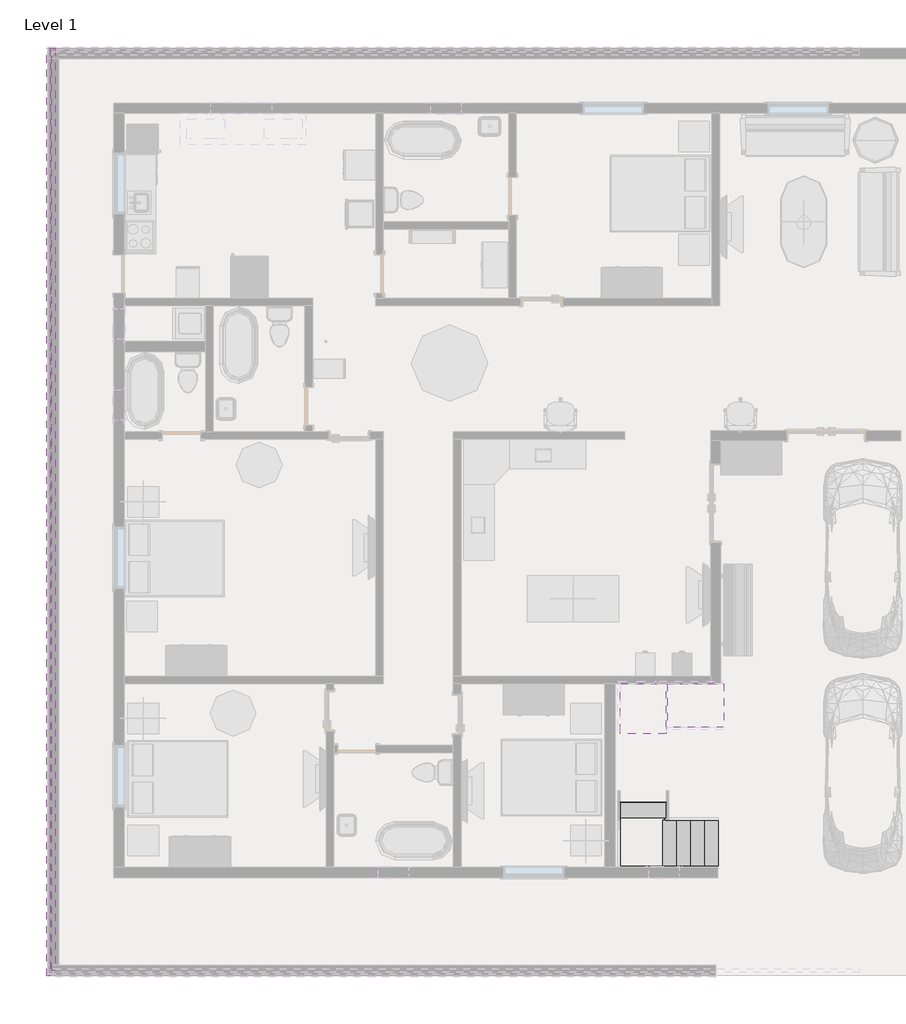
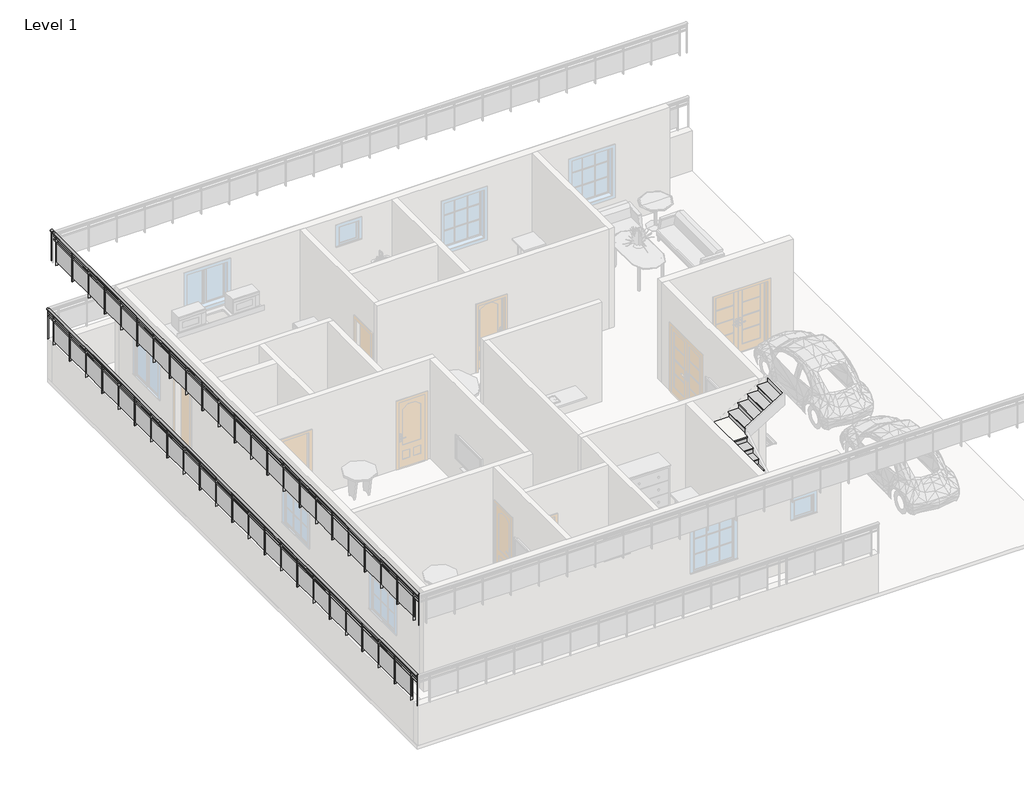
# One storey, part 3 of 6: 3 stair flights, 2 railings, 2 slabs.
"""IFC4 building model written with IfcOpenShell, lengths in millimetres."""

from ifc_helpers import new_model, si_unit, point, frame, origin, place, context, project, spatial, polyline, ellipse_curve, trimmed, outline, extrude, transform, mapped, element, save
from ifc_brep_helpers import plane_surface, extruded_surface, advanced_brep
from components import non_monolithic_landing_8bb0a33a, non_monolithic_landing_17065b0a, stair_flight_2df9e6b5, stair_flight_2e9a7ce1, stair_flight_c310d209

model = new_model("IFC4")

# Units and contexts
model_context = context("Model", 3, world=origin())
ifc_project = project(units=[si_unit("LENGTHUNIT", "METRE", prefix="MILLI")], contexts=[model_context])

# Site, building, storey
site = spatial("IfcSite", under=ifc_project)
building = spatial("IfcBuilding", under=site)
storey = spatial("IfcBuildingStorey", under=building, Name="Level 1", Elevation=0.0)

# Railings
placement = place(None, origin())
element("IfcRailing", 1, ObjectType="Glass Panel - Bottom Fill", at=placement, inside=storey, context=model_context, shape_type="SolidModel", body=[
    advanced_brep(
    [(-7851.6402326, 14000.8633056, 2133.6), (-7927.8402326, 14000.8633056, 2133.6), (-7851.6402326, -4490.3366944, 2133.6), (-7927.8402326, -4490.3366944, 2133.6)],
    [
        (0, 1, ellipse_curve(frame((-7889.7402326, 14000.8633056, 2133.6), z_axis=(0.0, 1.0, 0.0), x_axis=(-1.0, 0.0, 0.0)), 38.1, 28.575)),
        (1, 0, ellipse_curve(frame((-7889.7402326, 14000.8633056, 2133.6), z_axis=(0.0, 1.0, 0.0), x_axis=(-1.0, 0.0, 0.0)), 38.1, 28.575)),
        (2, 3, ellipse_curve(frame((-7889.7402326, -4490.3366944, 2133.6), z_axis=(0.0, -1.0, 0.0), x_axis=(-1.0, 0.0, 0.0)), 38.1, 28.575)),
        (3, 2, ellipse_curve(frame((-7889.7402326, -4490.3366944, 2133.6), z_axis=(0.0, -1.0, 0.0), x_axis=(-1.0, 0.0, 0.0)), 38.1, 28.575)),
        (0, 2),
        (3, 1),
    ],
    [
        plane_surface(frame((-7889.7402326, 14000.8633056, 2133.6), z_axis=(0.0, 1.0, 0.0), x_axis=(0.0, 0.0, -1.0))),
        plane_surface(frame((-7889.7402326, -4490.3366944, 2133.6), z_axis=(0.0, -1.0, 0.0), x_axis=(0.0, 0.0, -1.0))),
        extruded_surface(trimmed(ellipse_curve(frame((-7889.7402326, -4490.3366944, 2133.6), z_axis=(0.0, 1.0, 0.0), x_axis=(-1.0, 0.0, 0.0)), 38.1, 28.575), [point((-7851.6402326, -4490.3366944, 2133.6))], [point((-7927.8402326, -4490.3366944, 2133.6))], True, "CARTESIAN"), (0.0, 18491.2, 0.0), 18491.2),
        extruded_surface(trimmed(ellipse_curve(frame((-7889.7402326, -4490.3366944, 2133.6), z_axis=(0.0, 1.0, 0.0), x_axis=(-1.0, 0.0, 0.0)), 38.1, 28.575), [point((-7927.8402326, -4490.3366944, 2133.6))], [point((-7851.6402326, -4490.3366944, 2133.6))], True, "CARTESIAN"), (0.0, 18491.2, 0.0), 18491.2),
    ],
    [
        (0, [[1, 2]]),
        (1, [[3, 4]]),
        (2, [[-1, 5, -4, 6]]),
        (3, [[-2, -6, -3, -5]]),
    ],
),
    extrude(outline(polyline([(-7902.4402326, 14000.8633056), (-7877.0402326, 14000.8633056), (-7877.0402326, -4490.3366944), (-7902.4402326, -4490.3366944), (-7902.4402326, 14000.8633056)])), frame((0.0, 0.0, 2019.3), z_axis=(0.0, 0.0, 1.0), x_axis=(1.0, 0.0, 0.0)), (0.0, 0.0, 1.0), 25.4),
    extrude(outline(polyline([(-7902.4402326, 14000.8633056), (-7877.0402326, 14000.8633056), (-7877.0402326, -4490.3366944), (-7902.4402326, -4490.3366944), (-7902.4402326, 14000.8633056)])), frame((0.0, 0.0, 1917.7), z_axis=(0.0, 0.0, 1.0), x_axis=(1.0, 0.0, 0.0)), (0.0, 0.0, 1.0), 25.4),
    extrude(outline(polyline([(-7915.1402326, -4179.1866944), (-7864.3402326, -4179.1866944), (-7864.3402326, -4191.8866944), (-7915.1402326, -4191.8866944), (-7915.1402326, -4179.1866944)])), frame((0.0, 0.0, 1219.2), z_axis=(0.0, 0.0, 1.0), x_axis=(1.0, 0.0, 0.0)), (0.0, 0.0, 1.0), 885.6788223),
    extrude(outline(polyline([(-7883.2050756, -3372.7366944), (-7883.2050756, -4185.5366944), (-7889.5550756, -4185.5366944), (-7889.5550756, -3372.7366944), (-7883.2050756, -3372.7366944)])), frame((0.0, 0.0, 1320.8), z_axis=(0.0, 0.0, 1.0), x_axis=(1.0, 0.0, 0.0)), (0.0, 0.0, 1.0), 596.9),
    extrude(outline(polyline([(-7915.1402326, -3366.3866944), (-7864.3402326, -3366.3866944), (-7864.3402326, -3379.0866944), (-7915.1402326, -3379.0866944), (-7915.1402326, -3366.3866944)])), frame((0.0, 0.0, 1219.2), z_axis=(0.0, 0.0, 1.0), x_axis=(1.0, 0.0, 0.0)), (0.0, 0.0, 1.0), 885.6788223),
    extrude(outline(polyline([(-7883.2050756, -2559.9366944), (-7883.2050756, -3372.7366944), (-7889.5550756, -3372.7366944), (-7889.5550756, -2559.9366944), (-7883.2050756, -2559.9366944)])), frame((0.0, 0.0, 1320.8), z_axis=(0.0, 0.0, 1.0), x_axis=(1.0, 0.0, 0.0)), (0.0, 0.0, 1.0), 596.9),
    extrude(outline(polyline([(-7915.1402326, -2553.5866944), (-7864.3402326, -2553.5866944), (-7864.3402326, -2566.2866944), (-7915.1402326, -2566.2866944), (-7915.1402326, -2553.5866944)])), frame((0.0, 0.0, 1219.2), z_axis=(0.0, 0.0, 1.0), x_axis=(1.0, 0.0, 0.0)), (0.0, 0.0, 1.0), 885.6788223),
    extrude(outline(polyline([(-7883.2050756, -1747.1366944), (-7883.2050756, -2559.9366944), (-7889.5550756, -2559.9366944), (-7889.5550756, -1747.1366944), (-7883.2050756, -1747.1366944)])), frame((0.0, 0.0, 1320.8), z_axis=(0.0, 0.0, 1.0), x_axis=(1.0, 0.0, 0.0)), (0.0, 0.0, 1.0), 596.9),
    extrude(outline(polyline([(-7915.1402326, -1740.7866944), (-7864.3402326, -1740.7866944), (-7864.3402326, -1753.4866944), (-7915.1402326, -1753.4866944), (-7915.1402326, -1740.7866944)])), frame((0.0, 0.0, 1219.2), z_axis=(0.0, 0.0, 1.0), x_axis=(1.0, 0.0, 0.0)), (0.0, 0.0, 1.0), 885.6788223),
    extrude(outline(polyline([(-7883.2050756, -934.3366944), (-7883.2050756, -1747.1366944), (-7889.5550756, -1747.1366944), (-7889.5550756, -934.3366944), (-7883.2050756, -934.3366944)])), frame((0.0, 0.0, 1320.8), z_axis=(0.0, 0.0, 1.0), x_axis=(1.0, 0.0, 0.0)), (0.0, 0.0, 1.0), 596.9),
    extrude(outline(polyline([(-7915.1402326, -927.9866944), (-7864.3402326, -927.9866944), (-7864.3402326, -940.6866944), (-7915.1402326, -940.6866944), (-7915.1402326, -927.9866944)])), frame((0.0, 0.0, 1219.2), z_axis=(0.0, 0.0, 1.0), x_axis=(1.0, 0.0, 0.0)), (0.0, 0.0, 1.0), 885.6788223),
    extrude(outline(polyline([(-7883.2050756, -121.5366944), (-7883.2050756, -934.3366944), (-7889.5550756, -934.3366944), (-7889.5550756, -121.5366944), (-7883.2050756, -121.5366944)])), frame((0.0, 0.0, 1320.8), z_axis=(0.0, 0.0, 1.0), x_axis=(1.0, 0.0, 0.0)), (0.0, 0.0, 1.0), 596.9),
    extrude(outline(polyline([(-7915.1402326, -115.1866944), (-7864.3402326, -115.1866944), (-7864.3402326, -127.8866944), (-7915.1402326, -127.8866944), (-7915.1402326, -115.1866944)])), frame((0.0, 0.0, 1219.2), z_axis=(0.0, 0.0, 1.0), x_axis=(1.0, 0.0, 0.0)), (0.0, 0.0, 1.0), 885.6788223),
    extrude(outline(polyline([(-7883.2050756, 691.2633056), (-7883.2050756, -121.5366944), (-7889.5550756, -121.5366944), (-7889.5550756, 691.2633056), (-7883.2050756, 691.2633056)])), frame((0.0, 0.0, 1320.8), z_axis=(0.0, 0.0, 1.0), x_axis=(1.0, 0.0, 0.0)), (0.0, 0.0, 1.0), 596.9),
    extrude(outline(polyline([(-7915.1402326, 697.6133056), (-7864.3402326, 697.6133056), (-7864.3402326, 684.9133056), (-7915.1402326, 684.9133056), (-7915.1402326, 697.6133056)])), frame((0.0, 0.0, 1219.2), z_axis=(0.0, 0.0, 1.0), x_axis=(1.0, 0.0, 0.0)), (0.0, 0.0, 1.0), 885.6788223),
    extrude(outline(polyline([(-7883.2050756, 1504.0633056), (-7883.2050756, 691.2633056), (-7889.5550756, 691.2633056), (-7889.5550756, 1504.0633056), (-7883.2050756, 1504.0633056)])), frame((0.0, 0.0, 1320.8), z_axis=(0.0, 0.0, 1.0), x_axis=(1.0, 0.0, 0.0)), (0.0, 0.0, 1.0), 596.9),
    extrude(outline(polyline([(-7915.1402326, 1510.4133056), (-7864.3402326, 1510.4133056), (-7864.3402326, 1497.7133056), (-7915.1402326, 1497.7133056), (-7915.1402326, 1510.4133056)])), frame((0.0, 0.0, 1219.2), z_axis=(0.0, 0.0, 1.0), x_axis=(1.0, 0.0, 0.0)), (0.0, 0.0, 1.0), 885.6788223),
    extrude(outline(polyline([(-7883.2050756, 2316.8633056), (-7883.2050756, 1504.0633056), (-7889.5550756, 1504.0633056), (-7889.5550756, 2316.8633056), (-7883.2050756, 2316.8633056)])), frame((0.0, 0.0, 1320.8), z_axis=(0.0, 0.0, 1.0), x_axis=(1.0, 0.0, 0.0)), (0.0, 0.0, 1.0), 596.9),
    extrude(outline(polyline([(-7915.1402326, 2323.2133056), (-7864.3402326, 2323.2133056), (-7864.3402326, 2310.5133056), (-7915.1402326, 2310.5133056), (-7915.1402326, 2323.2133056)])), frame((0.0, 0.0, 1219.2), z_axis=(0.0, 0.0, 1.0), x_axis=(1.0, 0.0, 0.0)), (0.0, 0.0, 1.0), 885.6788223),
    extrude(outline(polyline([(-7883.2050756, 3129.6633056), (-7883.2050756, 2316.8633056), (-7889.5550756, 2316.8633056), (-7889.5550756, 3129.6633056), (-7883.2050756, 3129.6633056)])), frame((0.0, 0.0, 1320.8), z_axis=(0.0, 0.0, 1.0), x_axis=(1.0, 0.0, 0.0)), (0.0, 0.0, 1.0), 596.9),
    extrude(outline(polyline([(-7915.1402326, 3136.0133056), (-7864.3402326, 3136.0133056), (-7864.3402326, 3123.3133056), (-7915.1402326, 3123.3133056), (-7915.1402326, 3136.0133056)])), frame((0.0, 0.0, 1219.2), z_axis=(0.0, 0.0, 1.0), x_axis=(1.0, 0.0, 0.0)), (0.0, 0.0, 1.0), 885.6788223),
    extrude(outline(polyline([(-7883.2050756, 3942.4633056), (-7883.2050756, 3129.6633056), (-7889.5550756, 3129.6633056), (-7889.5550756, 3942.4633056), (-7883.2050756, 3942.4633056)])), frame((0.0, 0.0, 1320.8), z_axis=(0.0, 0.0, 1.0), x_axis=(1.0, 0.0, 0.0)), (0.0, 0.0, 1.0), 596.9),
    extrude(outline(polyline([(-7915.1402326, 3948.8133056), (-7864.3402326, 3948.8133056), (-7864.3402326, 3936.1133056), (-7915.1402326, 3936.1133056), (-7915.1402326, 3948.8133056)])), frame((0.0, 0.0, 1219.2), z_axis=(0.0, 0.0, 1.0), x_axis=(1.0, 0.0, 0.0)), (0.0, 0.0, 1.0), 885.6788223),
    extrude(outline(polyline([(-7883.2050756, 4755.2633056), (-7883.2050756, 3942.4633056), (-7889.5550756, 3942.4633056), (-7889.5550756, 4755.2633056), (-7883.2050756, 4755.2633056)])), frame((0.0, 0.0, 1320.8), z_axis=(0.0, 0.0, 1.0), x_axis=(1.0, 0.0, 0.0)), (0.0, 0.0, 1.0), 596.9),
    extrude(outline(polyline([(-7915.1402326, 4761.6133056), (-7864.3402326, 4761.6133056), (-7864.3402326, 4748.9133056), (-7915.1402326, 4748.9133056), (-7915.1402326, 4761.6133056)])), frame((0.0, 0.0, 1219.2), z_axis=(0.0, 0.0, 1.0), x_axis=(1.0, 0.0, 0.0)), (0.0, 0.0, 1.0), 885.6788223),
    extrude(outline(polyline([(-7883.2050756, 5568.0633056), (-7883.2050756, 4755.2633056), (-7889.5550756, 4755.2633056), (-7889.5550756, 5568.0633056), (-7883.2050756, 5568.0633056)])), frame((0.0, 0.0, 1320.8), z_axis=(0.0, 0.0, 1.0), x_axis=(1.0, 0.0, 0.0)), (0.0, 0.0, 1.0), 596.9),
    extrude(outline(polyline([(-7915.1402326, 5574.4133056), (-7864.3402326, 5574.4133056), (-7864.3402326, 5561.7133056), (-7915.1402326, 5561.7133056), (-7915.1402326, 5574.4133056)])), frame((0.0, 0.0, 1219.2), z_axis=(0.0, 0.0, 1.0), x_axis=(1.0, 0.0, 0.0)), (0.0, 0.0, 1.0), 885.6788223),
    extrude(outline(polyline([(-7883.2050756, 6380.8633056), (-7883.2050756, 5568.0633056), (-7889.5550756, 5568.0633056), (-7889.5550756, 6380.8633056), (-7883.2050756, 6380.8633056)])), frame((0.0, 0.0, 1320.8), z_axis=(0.0, 0.0, 1.0), x_axis=(1.0, 0.0, 0.0)), (0.0, 0.0, 1.0), 596.9),
    extrude(outline(polyline([(-7915.1402326, 6387.2133056), (-7864.3402326, 6387.2133056), (-7864.3402326, 6374.5133056), (-7915.1402326, 6374.5133056), (-7915.1402326, 6387.2133056)])), frame((0.0, 0.0, 1219.2), z_axis=(0.0, 0.0, 1.0), x_axis=(1.0, 0.0, 0.0)), (0.0, 0.0, 1.0), 885.6788223),
    extrude(outline(polyline([(-7883.2050756, 7193.6633056), (-7883.2050756, 6380.8633056), (-7889.5550756, 6380.8633056), (-7889.5550756, 7193.6633056), (-7883.2050756, 7193.6633056)])), frame((0.0, 0.0, 1320.8), z_axis=(0.0, 0.0, 1.0), x_axis=(1.0, 0.0, 0.0)), (0.0, 0.0, 1.0), 596.9),
    extrude(outline(polyline([(-7915.1402326, 7200.0133056), (-7864.3402326, 7200.0133056), (-7864.3402326, 7187.3133056), (-7915.1402326, 7187.3133056), (-7915.1402326, 7200.0133056)])), frame((0.0, 0.0, 1219.2), z_axis=(0.0, 0.0, 1.0), x_axis=(1.0, 0.0, 0.0)), (0.0, 0.0, 1.0), 885.6788223),
    extrude(outline(polyline([(-7883.2050756, 8006.4633056), (-7883.2050756, 7193.6633056), (-7889.5550756, 7193.6633056), (-7889.5550756, 8006.4633056), (-7883.2050756, 8006.4633056)])), frame((0.0, 0.0, 1320.8), z_axis=(0.0, 0.0, 1.0), x_axis=(1.0, 0.0, 0.0)), (0.0, 0.0, 1.0), 596.9),
    extrude(outline(polyline([(-7915.1402326, 8012.8133056), (-7864.3402326, 8012.8133056), (-7864.3402326, 8000.1133056), (-7915.1402326, 8000.1133056), (-7915.1402326, 8012.8133056)])), frame((0.0, 0.0, 1219.2), z_axis=(0.0, 0.0, 1.0), x_axis=(1.0, 0.0, 0.0)), (0.0, 0.0, 1.0), 885.6788223),
    extrude(outline(polyline([(-7883.2050756, 8819.2633056), (-7883.2050756, 8006.4633056), (-7889.5550756, 8006.4633056), (-7889.5550756, 8819.2633056), (-7883.2050756, 8819.2633056)])), frame((0.0, 0.0, 1320.8), z_axis=(0.0, 0.0, 1.0), x_axis=(1.0, 0.0, 0.0)), (0.0, 0.0, 1.0), 596.9),
    extrude(outline(polyline([(-7915.1402326, 8825.6133056), (-7864.3402326, 8825.6133056), (-7864.3402326, 8812.9133056), (-7915.1402326, 8812.9133056), (-7915.1402326, 8825.6133056)])), frame((0.0, 0.0, 1219.2), z_axis=(0.0, 0.0, 1.0), x_axis=(1.0, 0.0, 0.0)), (0.0, 0.0, 1.0), 885.6788223),
    extrude(outline(polyline([(-7883.2050756, 9632.0633056), (-7883.2050756, 8819.2633056), (-7889.5550756, 8819.2633056), (-7889.5550756, 9632.0633056), (-7883.2050756, 9632.0633056)])), frame((0.0, 0.0, 1320.8), z_axis=(0.0, 0.0, 1.0), x_axis=(1.0, 0.0, 0.0)), (0.0, 0.0, 1.0), 596.9),
    extrude(outline(polyline([(-7915.1402326, 9638.4133056), (-7864.3402326, 9638.4133056), (-7864.3402326, 9625.7133056), (-7915.1402326, 9625.7133056), (-7915.1402326, 9638.4133056)])), frame((0.0, 0.0, 1219.2), z_axis=(0.0, 0.0, 1.0), x_axis=(1.0, 0.0, 0.0)), (0.0, 0.0, 1.0), 885.6788223),
    extrude(outline(polyline([(-7883.2050756, 10444.8633056), (-7883.2050756, 9632.0633056), (-7889.5550756, 9632.0633056), (-7889.5550756, 10444.8633056), (-7883.2050756, 10444.8633056)])), frame((0.0, 0.0, 1320.8), z_axis=(0.0, 0.0, 1.0), x_axis=(1.0, 0.0, 0.0)), (0.0, 0.0, 1.0), 596.9),
    extrude(outline(polyline([(-7915.1402326, 10451.2133056), (-7864.3402326, 10451.2133056), (-7864.3402326, 10438.5133056), (-7915.1402326, 10438.5133056), (-7915.1402326, 10451.2133056)])), frame((0.0, 0.0, 1219.2), z_axis=(0.0, 0.0, 1.0), x_axis=(1.0, 0.0, 0.0)), (0.0, 0.0, 1.0), 885.6788223),
    extrude(outline(polyline([(-7883.2050756, 11257.6633056), (-7883.2050756, 10444.8633056), (-7889.5550756, 10444.8633056), (-7889.5550756, 11257.6633056), (-7883.2050756, 11257.6633056)])), frame((0.0, 0.0, 1320.8), z_axis=(0.0, 0.0, 1.0), x_axis=(1.0, 0.0, 0.0)), (0.0, 0.0, 1.0), 596.9),
    extrude(outline(polyline([(-7915.1402326, 11264.0133056), (-7864.3402326, 11264.0133056), (-7864.3402326, 11251.3133056), (-7915.1402326, 11251.3133056), (-7915.1402326, 11264.0133056)])), frame((0.0, 0.0, 1219.2), z_axis=(0.0, 0.0, 1.0), x_axis=(1.0, 0.0, 0.0)), (0.0, 0.0, 1.0), 885.6788223),
    extrude(outline(polyline([(-7883.2050756, 12070.4633056), (-7883.2050756, 11257.6633056), (-7889.5550756, 11257.6633056), (-7889.5550756, 12070.4633056), (-7883.2050756, 12070.4633056)])), frame((0.0, 0.0, 1320.8), z_axis=(0.0, 0.0, 1.0), x_axis=(1.0, 0.0, 0.0)), (0.0, 0.0, 1.0), 596.9),
    extrude(outline(polyline([(-7915.1402326, 12076.8133056), (-7864.3402326, 12076.8133056), (-7864.3402326, 12064.1133056), (-7915.1402326, 12064.1133056), (-7915.1402326, 12076.8133056)])), frame((0.0, 0.0, 1219.2), z_axis=(0.0, 0.0, 1.0), x_axis=(1.0, 0.0, 0.0)), (0.0, 0.0, 1.0), 885.6788223),
    extrude(outline(polyline([(-7883.2050756, 12883.2633056), (-7883.2050756, 12070.4633056), (-7889.5550756, 12070.4633056), (-7889.5550756, 12883.2633056), (-7883.2050756, 12883.2633056)])), frame((0.0, 0.0, 1320.8), z_axis=(0.0, 0.0, 1.0), x_axis=(1.0, 0.0, 0.0)), (0.0, 0.0, 1.0), 596.9),
    extrude(outline(polyline([(-7915.1402326, 12889.6133056), (-7864.3402326, 12889.6133056), (-7864.3402326, 12876.9133056), (-7915.1402326, 12876.9133056), (-7915.1402326, 12889.6133056)])), frame((0.0, 0.0, 1219.2), z_axis=(0.0, 0.0, 1.0), x_axis=(1.0, 0.0, 0.0)), (0.0, 0.0, 1.0), 885.6788223),
    extrude(outline(polyline([(-7883.2050756, 13696.0633056), (-7883.2050756, 12883.2633056), (-7889.5550756, 12883.2633056), (-7889.5550756, 13696.0633056), (-7883.2050756, 13696.0633056)])), frame((0.0, 0.0, 1320.8), z_axis=(0.0, 0.0, 1.0), x_axis=(1.0, 0.0, 0.0)), (0.0, 0.0, 1.0), 596.9),
    extrude(outline(polyline([(-7915.1402326, 13702.4133056), (-7864.3402326, 13702.4133056), (-7864.3402326, 13689.7133056), (-7915.1402326, 13689.7133056), (-7915.1402326, 13702.4133056)])), frame((0.0, 0.0, 1219.2), z_axis=(0.0, 0.0, 1.0), x_axis=(1.0, 0.0, 0.0)), (0.0, 0.0, 1.0), 885.6788223),
    extrude(outline(polyline([(-7899.2652326, -4477.6366944), (-7880.2152326, -4477.6366944), (-7880.2152326, -4496.6866944), (-7899.2652326, -4496.6866944), (-7899.2652326, -4477.6366944)])), frame((0.0, 0.0, 1219.2), z_axis=(0.0, 0.0, 1.0), x_axis=(1.0, 0.0, 0.0)), (0.0, 0.0, 1.0), 885.6788223),
    extrude(outline(polyline([(-7899.2652326, 14007.2133056), (-7880.2152326, 14007.2133056), (-7880.2152326, 13988.1633056), (-7899.2652326, 13988.1633056), (-7899.2652326, 14007.2133056)])), frame((0.0, 0.0, 1219.2), z_axis=(0.0, 0.0, 1.0), x_axis=(1.0, 0.0, 0.0)), (0.0, 0.0, 1.0), 885.6788223),
])
element("IfcRailing", 2, ObjectType="Glass Panel - Bottom Fill", at=placement, inside=storey, context=model_context, shape_type="SolidModel", body=[
    advanced_brep(
    [(-7750.0402326, 14000.8633056, 4495.8), (-7826.2402326, 14000.8633056, 4495.8), (-7750.0402326, -4388.7366944, 4495.8), (-7826.2402326, -4388.7366944, 4495.8)],
    [
        (0, 1, ellipse_curve(frame((-7788.1402326, 14000.8633056, 4495.8), z_axis=(0.0, 1.0, 0.0), x_axis=(-1.0, 0.0, 0.0)), 38.1, 28.575)),
        (1, 0, ellipse_curve(frame((-7788.1402326, 14000.8633056, 4495.8), z_axis=(0.0, 1.0, 0.0), x_axis=(-1.0, 0.0, 0.0)), 38.1, 28.575)),
        (2, 3, ellipse_curve(frame((-7788.1402326, -4388.7366944, 4495.8), z_axis=(0.0, -1.0, 0.0), x_axis=(-1.0, 0.0, 0.0)), 38.1, 28.575)),
        (3, 2, ellipse_curve(frame((-7788.1402326, -4388.7366944, 4495.8), z_axis=(0.0, -1.0, 0.0), x_axis=(-1.0, 0.0, 0.0)), 38.1, 28.575)),
        (0, 2),
        (3, 1),
    ],
    [
        plane_surface(frame((-7788.1402326, 14000.8633056, 4495.8), z_axis=(0.0, 1.0, 0.0), x_axis=(0.0, 0.0, -1.0))),
        plane_surface(frame((-7788.1402326, -4388.7366944, 4495.8), z_axis=(0.0, -1.0, 0.0), x_axis=(0.0, 0.0, -1.0))),
        extruded_surface(trimmed(ellipse_curve(frame((-7788.1402326, -4388.7366944, 4495.8), z_axis=(0.0, 1.0, 0.0), x_axis=(-1.0, 0.0, 0.0)), 38.1, 28.575), [point((-7750.0402326, -4388.7366944, 4495.8))], [point((-7826.2402326, -4388.7366944, 4495.8))], True, "CARTESIAN"), (0.0, 18389.6, 0.0), 18389.6),
        extruded_surface(trimmed(ellipse_curve(frame((-7788.1402326, -4388.7366944, 4495.8), z_axis=(0.0, 1.0, 0.0), x_axis=(-1.0, 0.0, 0.0)), 38.1, 28.575), [point((-7826.2402326, -4388.7366944, 4495.8))], [point((-7750.0402326, -4388.7366944, 4495.8))], True, "CARTESIAN"), (0.0, 18389.6, 0.0), 18389.6),
    ],
    [
        (0, [[1, 2]]),
        (1, [[3, 4]]),
        (2, [[-1, 5, -4, 6]]),
        (3, [[-2, -6, -3, -5]]),
    ],
),
    extrude(outline(polyline([(-7800.8402326, 14000.8633056), (-7775.4402326, 14000.8633056), (-7775.4402326, -4388.7366944), (-7800.8402326, -4388.7366944), (-7800.8402326, 14000.8633056)])), frame((0.0, 0.0, 4381.5), z_axis=(0.0, 0.0, 1.0), x_axis=(1.0, 0.0, 0.0)), (0.0, 0.0, 1.0), 25.4),
    extrude(outline(polyline([(-7800.8402326, 14000.8633056), (-7775.4402326, 14000.8633056), (-7775.4402326, -4388.7366944), (-7800.8402326, -4388.7366944), (-7800.8402326, 14000.8633056)])), frame((0.0, 0.0, 4279.9), z_axis=(0.0, 0.0, 1.0), x_axis=(1.0, 0.0, 0.0)), (0.0, 0.0, 1.0), 25.4),
    extrude(outline(polyline([(-7813.5402326, -4128.3866944), (-7762.7402326, -4128.3866944), (-7762.7402326, -4141.0866944), (-7813.5402326, -4141.0866944), (-7813.5402326, -4128.3866944)])), frame((0.0, 0.0, 3581.4), z_axis=(0.0, 0.0, 1.0), x_axis=(1.0, 0.0, 0.0)), (0.0, 0.0, 1.0), 885.6788223),
    extrude(outline(polyline([(-7781.6050756, -3321.9366944), (-7781.6050756, -4134.7366944), (-7787.9550756, -4134.7366944), (-7787.9550756, -3321.9366944), (-7781.6050756, -3321.9366944)])), frame((0.0, 0.0, 3683.0), z_axis=(0.0, 0.0, 1.0), x_axis=(1.0, 0.0, 0.0)), (0.0, 0.0, 1.0), 596.9),
    extrude(outline(polyline([(-7813.5402326, -3315.5866944), (-7762.7402326, -3315.5866944), (-7762.7402326, -3328.2866944), (-7813.5402326, -3328.2866944), (-7813.5402326, -3315.5866944)])), frame((0.0, 0.0, 3581.4), z_axis=(0.0, 0.0, 1.0), x_axis=(1.0, 0.0, 0.0)), (0.0, 0.0, 1.0), 885.6788223),
    extrude(outline(polyline([(-7781.6050756, -2509.1366944), (-7781.6050756, -3321.9366944), (-7787.9550756, -3321.9366944), (-7787.9550756, -2509.1366944), (-7781.6050756, -2509.1366944)])), frame((0.0, 0.0, 3683.0), z_axis=(0.0, 0.0, 1.0), x_axis=(1.0, 0.0, 0.0)), (0.0, 0.0, 1.0), 596.9),
    extrude(outline(polyline([(-7813.5402326, -2502.7866944), (-7762.7402326, -2502.7866944), (-7762.7402326, -2515.4866944), (-7813.5402326, -2515.4866944), (-7813.5402326, -2502.7866944)])), frame((0.0, 0.0, 3581.4), z_axis=(0.0, 0.0, 1.0), x_axis=(1.0, 0.0, 0.0)), (0.0, 0.0, 1.0), 885.6788223),
    extrude(outline(polyline([(-7781.6050756, -1696.3366944), (-7781.6050756, -2509.1366944), (-7787.9550756, -2509.1366944), (-7787.9550756, -1696.3366944), (-7781.6050756, -1696.3366944)])), frame((0.0, 0.0, 3683.0), z_axis=(0.0, 0.0, 1.0), x_axis=(1.0, 0.0, 0.0)), (0.0, 0.0, 1.0), 596.9),
    extrude(outline(polyline([(-7813.5402326, -1689.9866944), (-7762.7402326, -1689.9866944), (-7762.7402326, -1702.6866944), (-7813.5402326, -1702.6866944), (-7813.5402326, -1689.9866944)])), frame((0.0, 0.0, 3581.4), z_axis=(0.0, 0.0, 1.0), x_axis=(1.0, 0.0, 0.0)), (0.0, 0.0, 1.0), 885.6788223),
    extrude(outline(polyline([(-7781.6050756, -883.5366944), (-7781.6050756, -1696.3366944), (-7787.9550756, -1696.3366944), (-7787.9550756, -883.5366944), (-7781.6050756, -883.5366944)])), frame((0.0, 0.0, 3683.0), z_axis=(0.0, 0.0, 1.0), x_axis=(1.0, 0.0, 0.0)), (0.0, 0.0, 1.0), 596.9),
    extrude(outline(polyline([(-7813.5402326, -877.1866944), (-7762.7402326, -877.1866944), (-7762.7402326, -889.8866944), (-7813.5402326, -889.8866944), (-7813.5402326, -877.1866944)])), frame((0.0, 0.0, 3581.4), z_axis=(0.0, 0.0, 1.0), x_axis=(1.0, 0.0, 0.0)), (0.0, 0.0, 1.0), 885.6788223),
    extrude(outline(polyline([(-7781.6050756, -70.7366944), (-7781.6050756, -883.5366944), (-7787.9550756, -883.5366944), (-7787.9550756, -70.7366944), (-7781.6050756, -70.7366944)])), frame((0.0, 0.0, 3683.0), z_axis=(0.0, 0.0, 1.0), x_axis=(1.0, 0.0, 0.0)), (0.0, 0.0, 1.0), 596.9),
    extrude(outline(polyline([(-7813.5402326, -64.3866944), (-7762.7402326, -64.3866944), (-7762.7402326, -77.0866944), (-7813.5402326, -77.0866944), (-7813.5402326, -64.3866944)])), frame((0.0, 0.0, 3581.4), z_axis=(0.0, 0.0, 1.0), x_axis=(1.0, 0.0, 0.0)), (0.0, 0.0, 1.0), 885.6788223),
    extrude(outline(polyline([(-7781.6050756, 742.0633056), (-7781.6050756, -70.7366944), (-7787.9550756, -70.7366944), (-7787.9550756, 742.0633056), (-7781.6050756, 742.0633056)])), frame((0.0, 0.0, 3683.0), z_axis=(0.0, 0.0, 1.0), x_axis=(1.0, 0.0, 0.0)), (0.0, 0.0, 1.0), 596.9),
    extrude(outline(polyline([(-7813.5402326, 748.4133056), (-7762.7402326, 748.4133056), (-7762.7402326, 735.7133056), (-7813.5402326, 735.7133056), (-7813.5402326, 748.4133056)])), frame((0.0, 0.0, 3581.4), z_axis=(0.0, 0.0, 1.0), x_axis=(1.0, 0.0, 0.0)), (0.0, 0.0, 1.0), 885.6788223),
    extrude(outline(polyline([(-7781.6050756, 1554.8633056), (-7781.6050756, 742.0633056), (-7787.9550756, 742.0633056), (-7787.9550756, 1554.8633056), (-7781.6050756, 1554.8633056)])), frame((0.0, 0.0, 3683.0), z_axis=(0.0, 0.0, 1.0), x_axis=(1.0, 0.0, 0.0)), (0.0, 0.0, 1.0), 596.9),
    extrude(outline(polyline([(-7813.5402326, 1561.2133056), (-7762.7402326, 1561.2133056), (-7762.7402326, 1548.5133056), (-7813.5402326, 1548.5133056), (-7813.5402326, 1561.2133056)])), frame((0.0, 0.0, 3581.4), z_axis=(0.0, 0.0, 1.0), x_axis=(1.0, 0.0, 0.0)), (0.0, 0.0, 1.0), 885.6788223),
    extrude(outline(polyline([(-7781.6050756, 2367.6633056), (-7781.6050756, 1554.8633056), (-7787.9550756, 1554.8633056), (-7787.9550756, 2367.6633056), (-7781.6050756, 2367.6633056)])), frame((0.0, 0.0, 3683.0), z_axis=(0.0, 0.0, 1.0), x_axis=(1.0, 0.0, 0.0)), (0.0, 0.0, 1.0), 596.9),
    extrude(outline(polyline([(-7813.5402326, 2374.0133056), (-7762.7402326, 2374.0133056), (-7762.7402326, 2361.3133056), (-7813.5402326, 2361.3133056), (-7813.5402326, 2374.0133056)])), frame((0.0, 0.0, 3581.4), z_axis=(0.0, 0.0, 1.0), x_axis=(1.0, 0.0, 0.0)), (0.0, 0.0, 1.0), 885.6788223),
    extrude(outline(polyline([(-7781.6050756, 3180.4633056), (-7781.6050756, 2367.6633056), (-7787.9550756, 2367.6633056), (-7787.9550756, 3180.4633056), (-7781.6050756, 3180.4633056)])), frame((0.0, 0.0, 3683.0), z_axis=(0.0, 0.0, 1.0), x_axis=(1.0, 0.0, 0.0)), (0.0, 0.0, 1.0), 596.9),
    extrude(outline(polyline([(-7813.5402326, 3186.8133056), (-7762.7402326, 3186.8133056), (-7762.7402326, 3174.1133056), (-7813.5402326, 3174.1133056), (-7813.5402326, 3186.8133056)])), frame((0.0, 0.0, 3581.4), z_axis=(0.0, 0.0, 1.0), x_axis=(1.0, 0.0, 0.0)), (0.0, 0.0, 1.0), 885.6788223),
    extrude(outline(polyline([(-7781.6050756, 3993.2633056), (-7781.6050756, 3180.4633056), (-7787.9550756, 3180.4633056), (-7787.9550756, 3993.2633056), (-7781.6050756, 3993.2633056)])), frame((0.0, 0.0, 3683.0), z_axis=(0.0, 0.0, 1.0), x_axis=(1.0, 0.0, 0.0)), (0.0, 0.0, 1.0), 596.9),
    extrude(outline(polyline([(-7813.5402326, 3999.6133056), (-7762.7402326, 3999.6133056), (-7762.7402326, 3986.9133056), (-7813.5402326, 3986.9133056), (-7813.5402326, 3999.6133056)])), frame((0.0, 0.0, 3581.4), z_axis=(0.0, 0.0, 1.0), x_axis=(1.0, 0.0, 0.0)), (0.0, 0.0, 1.0), 885.6788223),
    extrude(outline(polyline([(-7781.6050756, 4806.0633056), (-7781.6050756, 3993.2633056), (-7787.9550756, 3993.2633056), (-7787.9550756, 4806.0633056), (-7781.6050756, 4806.0633056)])), frame((0.0, 0.0, 3683.0), z_axis=(0.0, 0.0, 1.0), x_axis=(1.0, 0.0, 0.0)), (0.0, 0.0, 1.0), 596.9),
    extrude(outline(polyline([(-7813.5402326, 4812.4133056), (-7762.7402326, 4812.4133056), (-7762.7402326, 4799.7133056), (-7813.5402326, 4799.7133056), (-7813.5402326, 4812.4133056)])), frame((0.0, 0.0, 3581.4), z_axis=(0.0, 0.0, 1.0), x_axis=(1.0, 0.0, 0.0)), (0.0, 0.0, 1.0), 885.6788223),
    extrude(outline(polyline([(-7781.6050756, 5618.8633056), (-7781.6050756, 4806.0633056), (-7787.9550756, 4806.0633056), (-7787.9550756, 5618.8633056), (-7781.6050756, 5618.8633056)])), frame((0.0, 0.0, 3683.0), z_axis=(0.0, 0.0, 1.0), x_axis=(1.0, 0.0, 0.0)), (0.0, 0.0, 1.0), 596.9),
    extrude(outline(polyline([(-7813.5402326, 5625.2133056), (-7762.7402326, 5625.2133056), (-7762.7402326, 5612.5133056), (-7813.5402326, 5612.5133056), (-7813.5402326, 5625.2133056)])), frame((0.0, 0.0, 3581.4), z_axis=(0.0, 0.0, 1.0), x_axis=(1.0, 0.0, 0.0)), (0.0, 0.0, 1.0), 885.6788223),
    extrude(outline(polyline([(-7781.6050756, 6431.6633056), (-7781.6050756, 5618.8633056), (-7787.9550756, 5618.8633056), (-7787.9550756, 6431.6633056), (-7781.6050756, 6431.6633056)])), frame((0.0, 0.0, 3683.0), z_axis=(0.0, 0.0, 1.0), x_axis=(1.0, 0.0, 0.0)), (0.0, 0.0, 1.0), 596.9),
    extrude(outline(polyline([(-7813.5402326, 6438.0133056), (-7762.7402326, 6438.0133056), (-7762.7402326, 6425.3133056), (-7813.5402326, 6425.3133056), (-7813.5402326, 6438.0133056)])), frame((0.0, 0.0, 3581.4), z_axis=(0.0, 0.0, 1.0), x_axis=(1.0, 0.0, 0.0)), (0.0, 0.0, 1.0), 885.6788223),
    extrude(outline(polyline([(-7781.6050756, 7244.4633056), (-7781.6050756, 6431.6633056), (-7787.9550756, 6431.6633056), (-7787.9550756, 7244.4633056), (-7781.6050756, 7244.4633056)])), frame((0.0, 0.0, 3683.0), z_axis=(0.0, 0.0, 1.0), x_axis=(1.0, 0.0, 0.0)), (0.0, 0.0, 1.0), 596.9),
    extrude(outline(polyline([(-7813.5402326, 7250.8133056), (-7762.7402326, 7250.8133056), (-7762.7402326, 7238.1133056), (-7813.5402326, 7238.1133056), (-7813.5402326, 7250.8133056)])), frame((0.0, 0.0, 3581.4), z_axis=(0.0, 0.0, 1.0), x_axis=(1.0, 0.0, 0.0)), (0.0, 0.0, 1.0), 885.6788223),
    extrude(outline(polyline([(-7781.6050756, 8057.2633056), (-7781.6050756, 7244.4633056), (-7787.9550756, 7244.4633056), (-7787.9550756, 8057.2633056), (-7781.6050756, 8057.2633056)])), frame((0.0, 0.0, 3683.0), z_axis=(0.0, 0.0, 1.0), x_axis=(1.0, 0.0, 0.0)), (0.0, 0.0, 1.0), 596.9),
    extrude(outline(polyline([(-7813.5402326, 8063.6133056), (-7762.7402326, 8063.6133056), (-7762.7402326, 8050.9133056), (-7813.5402326, 8050.9133056), (-7813.5402326, 8063.6133056)])), frame((0.0, 0.0, 3581.4), z_axis=(0.0, 0.0, 1.0), x_axis=(1.0, 0.0, 0.0)), (0.0, 0.0, 1.0), 885.6788223),
    extrude(outline(polyline([(-7781.6050756, 8870.0633056), (-7781.6050756, 8057.2633056), (-7787.9550756, 8057.2633056), (-7787.9550756, 8870.0633056), (-7781.6050756, 8870.0633056)])), frame((0.0, 0.0, 3683.0), z_axis=(0.0, 0.0, 1.0), x_axis=(1.0, 0.0, 0.0)), (0.0, 0.0, 1.0), 596.9),
    extrude(outline(polyline([(-7813.5402326, 8876.4133056), (-7762.7402326, 8876.4133056), (-7762.7402326, 8863.7133056), (-7813.5402326, 8863.7133056), (-7813.5402326, 8876.4133056)])), frame((0.0, 0.0, 3581.4), z_axis=(0.0, 0.0, 1.0), x_axis=(1.0, 0.0, 0.0)), (0.0, 0.0, 1.0), 885.6788223),
    extrude(outline(polyline([(-7781.6050756, 9682.8633056), (-7781.6050756, 8870.0633056), (-7787.9550756, 8870.0633056), (-7787.9550756, 9682.8633056), (-7781.6050756, 9682.8633056)])), frame((0.0, 0.0, 3683.0), z_axis=(0.0, 0.0, 1.0), x_axis=(1.0, 0.0, 0.0)), (0.0, 0.0, 1.0), 596.9),
    extrude(outline(polyline([(-7813.5402326, 9689.2133056), (-7762.7402326, 9689.2133056), (-7762.7402326, 9676.5133056), (-7813.5402326, 9676.5133056), (-7813.5402326, 9689.2133056)])), frame((0.0, 0.0, 3581.4), z_axis=(0.0, 0.0, 1.0), x_axis=(1.0, 0.0, 0.0)), (0.0, 0.0, 1.0), 885.6788223),
    extrude(outline(polyline([(-7781.6050756, 10495.6633056), (-7781.6050756, 9682.8633056), (-7787.9550756, 9682.8633056), (-7787.9550756, 10495.6633056), (-7781.6050756, 10495.6633056)])), frame((0.0, 0.0, 3683.0), z_axis=(0.0, 0.0, 1.0), x_axis=(1.0, 0.0, 0.0)), (0.0, 0.0, 1.0), 596.9),
    extrude(outline(polyline([(-7813.5402326, 10502.0133056), (-7762.7402326, 10502.0133056), (-7762.7402326, 10489.3133056), (-7813.5402326, 10489.3133056), (-7813.5402326, 10502.0133056)])), frame((0.0, 0.0, 3581.4), z_axis=(0.0, 0.0, 1.0), x_axis=(1.0, 0.0, 0.0)), (0.0, 0.0, 1.0), 885.6788223),
    extrude(outline(polyline([(-7781.6050756, 11308.4633056), (-7781.6050756, 10495.6633056), (-7787.9550756, 10495.6633056), (-7787.9550756, 11308.4633056), (-7781.6050756, 11308.4633056)])), frame((0.0, 0.0, 3683.0), z_axis=(0.0, 0.0, 1.0), x_axis=(1.0, 0.0, 0.0)), (0.0, 0.0, 1.0), 596.9),
    extrude(outline(polyline([(-7813.5402326, 11314.8133056), (-7762.7402326, 11314.8133056), (-7762.7402326, 11302.1133056), (-7813.5402326, 11302.1133056), (-7813.5402326, 11314.8133056)])), frame((0.0, 0.0, 3581.4), z_axis=(0.0, 0.0, 1.0), x_axis=(1.0, 0.0, 0.0)), (0.0, 0.0, 1.0), 885.6788223),
    extrude(outline(polyline([(-7781.6050756, 12121.2633056), (-7781.6050756, 11308.4633056), (-7787.9550756, 11308.4633056), (-7787.9550756, 12121.2633056), (-7781.6050756, 12121.2633056)])), frame((0.0, 0.0, 3683.0), z_axis=(0.0, 0.0, 1.0), x_axis=(1.0, 0.0, 0.0)), (0.0, 0.0, 1.0), 596.9),
    extrude(outline(polyline([(-7813.5402326, 12127.6133056), (-7762.7402326, 12127.6133056), (-7762.7402326, 12114.9133056), (-7813.5402326, 12114.9133056), (-7813.5402326, 12127.6133056)])), frame((0.0, 0.0, 3581.4), z_axis=(0.0, 0.0, 1.0), x_axis=(1.0, 0.0, 0.0)), (0.0, 0.0, 1.0), 885.6788223),
    extrude(outline(polyline([(-7781.6050756, 12934.0633056), (-7781.6050756, 12121.2633056), (-7787.9550756, 12121.2633056), (-7787.9550756, 12934.0633056), (-7781.6050756, 12934.0633056)])), frame((0.0, 0.0, 3683.0), z_axis=(0.0, 0.0, 1.0), x_axis=(1.0, 0.0, 0.0)), (0.0, 0.0, 1.0), 596.9),
    extrude(outline(polyline([(-7813.5402326, 12940.4133056), (-7762.7402326, 12940.4133056), (-7762.7402326, 12927.7133056), (-7813.5402326, 12927.7133056), (-7813.5402326, 12940.4133056)])), frame((0.0, 0.0, 3581.4), z_axis=(0.0, 0.0, 1.0), x_axis=(1.0, 0.0, 0.0)), (0.0, 0.0, 1.0), 885.6788223),
    extrude(outline(polyline([(-7781.6050756, 13746.8633056), (-7781.6050756, 12934.0633056), (-7787.9550756, 12934.0633056), (-7787.9550756, 13746.8633056), (-7781.6050756, 13746.8633056)])), frame((0.0, 0.0, 3683.0), z_axis=(0.0, 0.0, 1.0), x_axis=(1.0, 0.0, 0.0)), (0.0, 0.0, 1.0), 596.9),
    extrude(outline(polyline([(-7813.5402326, 13753.2133056), (-7762.7402326, 13753.2133056), (-7762.7402326, 13740.5133056), (-7813.5402326, 13740.5133056), (-7813.5402326, 13753.2133056)])), frame((0.0, 0.0, 3581.4), z_axis=(0.0, 0.0, 1.0), x_axis=(1.0, 0.0, 0.0)), (0.0, 0.0, 1.0), 885.6788223),
    extrude(outline(polyline([(-7797.6652326, -4376.0366944), (-7778.6152326, -4376.0366944), (-7778.6152326, -4395.0866944), (-7797.6652326, -4395.0866944), (-7797.6652326, -4376.0366944)])), frame((0.0, 0.0, 3581.4), z_axis=(0.0, 0.0, 1.0), x_axis=(1.0, 0.0, 0.0)), (0.0, 0.0, 1.0), 885.6788223),
    extrude(outline(polyline([(-7797.6652326, 14007.2133056), (-7778.6152326, 14007.2133056), (-7778.6152326, 13988.1633056), (-7797.6652326, 13988.1633056), (-7797.6652326, 14007.2133056)])), frame((0.0, 0.0, 3581.4), z_axis=(0.0, 0.0, 1.0), x_axis=(1.0, 0.0, 0.0)), (0.0, 0.0, 1.0), 885.6788223),
])

# Slabs
non_monolithic_landing_shape = non_monolithic_landing_8bb0a33a(model_context)
element("IfcSlab", 3, ObjectType="Non-Monolithic Landing", at=placement, inside=storey, context=model_context, shape_type="MappedRepresentation", body=[
    mapped(non_monolithic_landing_shape, transform((0.0, 0.0, 0.0), x_axis=(1.0, 0.0, 0.0), y_axis=(0.0, 1.0, 0.0), z_axis=(0.0, 0.0, 1.0))),
])
non_monolithic_landing_2_shape = non_monolithic_landing_17065b0a(model_context)
element("IfcSlab", 4, ObjectType="Non-Monolithic Landing", at=placement, inside=storey, context=model_context, shape_type="MappedRepresentation", body=[
    mapped(non_monolithic_landing_2_shape, transform((0.0, 0.0, 0.0), x_axis=(1.0, 0.0, 0.0), y_axis=(0.0, 1.0, 0.0), z_axis=(0.0, 0.0, 1.0))),
])

# Stair flights
stair_flight_shape = stair_flight_2df9e6b5(model_context)
element("IfcStairFlight", 5, ObjectType="2\" Tread 1\" Nosing 1/4\" Riser", at=placement, inside=storey, context=model_context, shape_type="MappedRepresentation", body=[
    mapped(stair_flight_shape, transform((0.0, 0.0, 0.0), x_axis=(1.0, 0.0, 0.0), y_axis=(0.0, 1.0, 0.0), z_axis=(0.0, 0.0, 1.0))),
])
stair_flight_2_shape = stair_flight_2e9a7ce1(model_context)
element("IfcStairFlight", 6, ObjectType="2\" Tread 1\" Nosing 1/4\" Riser", at=placement, inside=storey, context=model_context, shape_type="MappedRepresentation", body=[
    mapped(stair_flight_2_shape, transform((0.0, 0.0, 0.0), x_axis=(1.0, 0.0, 0.0), y_axis=(0.0, 1.0, 0.0), z_axis=(0.0, 0.0, 1.0))),
])
stair_flight_3_shape = stair_flight_c310d209(model_context)
element("IfcStairFlight", 7, ObjectType="2\" Tread 1\" Nosing 1/4\" Riser", at=placement, inside=storey, context=model_context, shape_type="MappedRepresentation", body=[
    mapped(stair_flight_3_shape, transform((0.0, 0.0, 0.0), x_axis=(1.0, 0.0, 0.0), y_axis=(0.0, 1.0, 0.0), z_axis=(0.0, 0.0, 1.0))),
])

save(model, "model.ifc")

# Revit data of these elements
# Type "Glass Panel - Bottom Fill"
#   Assembly Code = "C2010400"
#   built-in parameter 1008612 = 0.0416667 (stored number, unit not read)
#   built-in parameter 1008611 = 0.0416667 (stored number, unit not read)
#   built-in parameter 1008609 = 0.333333 (stored number, unit not read)
#   built-in parameter 1008604 = 0.166667 (stored number, unit not read)
#   built-in parameter 1008603 = 0.166667 (stored number, unit not read)
#   Railing Height = 3' - 0"
#   built-in parameter 1008630 = 2
#   built-in parameter 1008610 = 2
#   built-in parameter 1008618 = Baluster - Square : 3/4"
# Element 1 (IfcRailing, "Glass Panel - Bottom Fill")
#   built-in parameter 1008621 = 4 (stored number, unit not read)
#   Phase Created = New Construction
#   Materials on its faces: "Glass"
# Element 2 (IfcRailing, "Glass Panel - Bottom Fill")
#   built-in parameter 1008621 = 11.75 (stored number, unit not read)
#   Phase Created = New Construction
#   Materials on its faces: "Glass"
# Elements 3, 4 (IfcSlab, "Non-Monolithic Landing")
#   Phase Created = New Construction
# Elements 5, 6, 7 (IfcStairFlight, "2\" Tread 1\" Nosing 1/4\" Riser")
#   Phase Created = New Construction
# Materials
#   "Glass": class "Glass", colour RGB 0 128 192, transparency 0.75, Description = "Soda Lime Glass", Cost = 0
